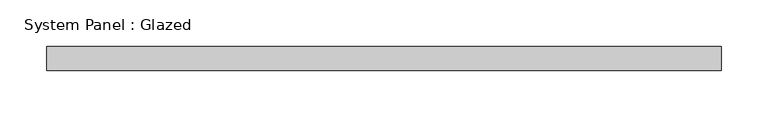
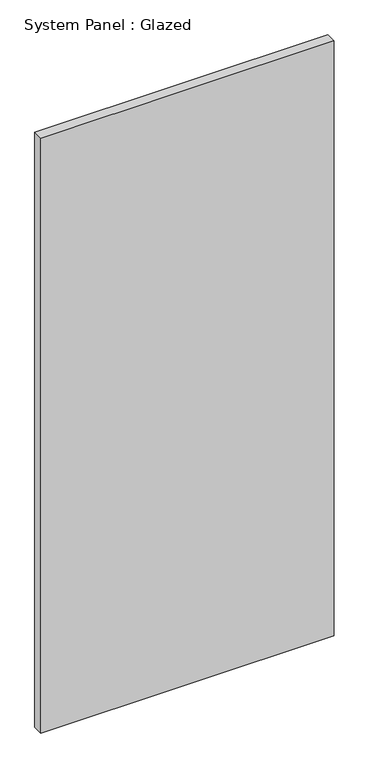
"""IFC4 building model written with IfcOpenShell, lengths in millimetres: plate geometry, System Panel : Glazed."""

from ifc_helpers import new_model, si_unit, origin, origin_with_axes, place, context, project, spatial, polyline, outline, extrude, source, transform, mapped, element, save


def system_panel_glazed_bd259d29(model_context):
    return source(origin(), model_context, "Body", "SweptSolid", [
        extrude(outline(polyline([(358.775, 19.05), (-358.775, 19.05), (-358.775, 44.45), (358.775, 44.45), (358.775, 19.05)])), origin_with_axes(), (0.0, 0.0, 1.0), 1538.799372),
    ])


if __name__ == "__main__":
    model = new_model("IFC4")
    model_context = context("Model", 3, world=origin())
    ifc_project = project(units=[si_unit("LENGTHUNIT", "METRE", prefix="MILLI")], contexts=[model_context])
    site = spatial("IfcSite", under=ifc_project)
    building = spatial("IfcBuilding", under=site)
    placement = place(None, origin())
    system_panel_glazed_shape = system_panel_glazed_bd259d29(model_context)
    element("IfcPlate", 1, ObjectType="System Panel : Glazed", at=placement, inside=building, context=model_context, shape_type="MappedRepresentation", body=[
        mapped(system_panel_glazed_shape, transform((0.0, 0.0, 0.0), x_axis=(1.0, 0.0, 0.0), y_axis=(0.0, 1.0, 0.0), z_axis=(0.0, 0.0, 1.0))),
    ])
    save(model, "model.ifc")

# Revit data of these elements
# Type "System Panel : Glazed"
#   Construction Type Id = "GSP4R"
#   Analytic Construction = "1/8 in Pilkington single glazing"
#   Visual Light Transmittance = 0.9
#   Solar Heat Gain Coefficient = 0.86
#   Heat Transfer Coefficient (U) = 1.18115 BTU/(h·ft²·°F)
#   Define Thermal Properties by = 1
# Element 1 (IfcPlate, "System Panel : Glazed")
#   Materials on its faces: "Glass"
# Materials
#   "Glass": class "Glass", colour RGB 0 128 192, transparency 0.75, Description = "Soda Lime Glass", Cost = 0
